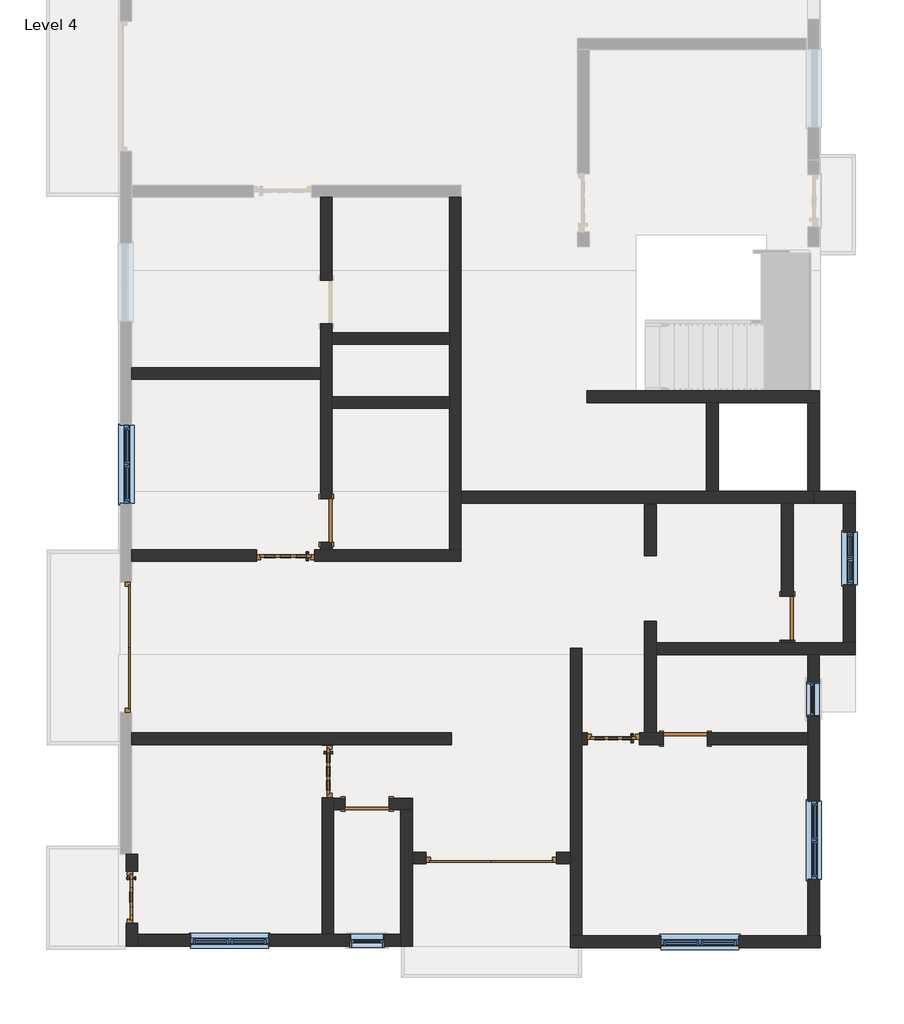
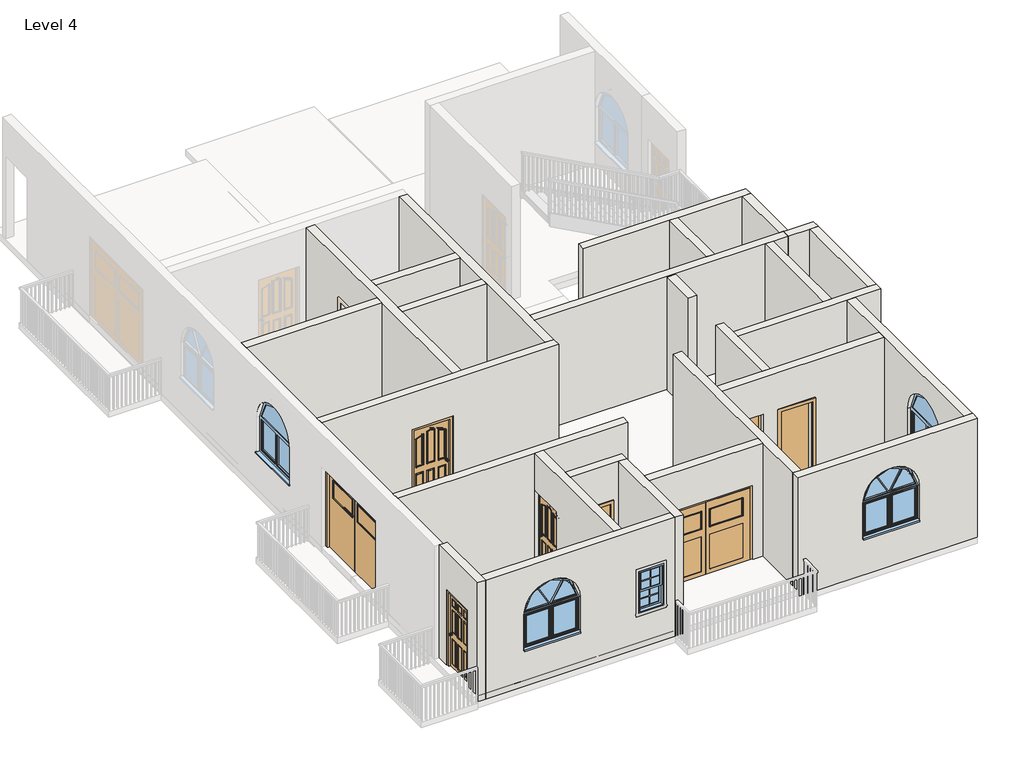
# One storey, part 1 of 7: 27 walls, 10 doors, 7 windows.
"""IFC4 building model written with IfcOpenShell, lengths in millimetres."""

from ifc_helpers import new_model, si_unit, frame, origin, place, context, project, spatial, polyline, circle_curve, outline, extrude, faceted_brep, transform, mapped, element, save
from ifc_brep_helpers import plane_surface, revolved_surface, advanced_brep
from components import doors_extsgl_5_910x2110mm_99758a98, doors_extsgl_6_1010x2110mm_b93c615f, doors_extsgl_6_1010x2110mm_efbaf1af, doors_extsgl_6_910x2110mm_72be2df1, doors_extsgl_6_910x2110mm_b26fcae4, doors_extsgl_6_910x2110mm_5dc58899, doors_extsgl_6_910x2110mm_16d7c084, doors_garage_timber_side_hung_glazing_2270x2050mm_ae99176d, doors_garage_timber_side_hung_glazing_2270x2200mm_badb7014, door_fadea3f2, door_53b1b562, window_679d2811, windows_arched_1360x910mm_c5754810, windows_dbl_w_glazing_bars_910x910mm_41eba874

model = new_model("IFC4")

# Units and contexts
model_context = context("Model", 3, world=origin())
ifc_project = project(units=[si_unit("LENGTHUNIT", "METRE", prefix="MILLI")], contexts=[model_context])

# Site, building, storey
site = spatial("IfcSite", under=ifc_project)
building = spatial("IfcBuilding", under=site)
storey = spatial("IfcBuildingStorey", under=building, Name="Level 4", Elevation=9144.0)

# Doors
placement = place(None, origin())
doors_extsgl_5_910x2110mm_shape = doors_extsgl_5_910x2110mm_99758a98(model_context)
element("IfcDoor", 1, ObjectType="Doors_ExtSgl_5 : 910x2110mm", at=placement, inside=storey, context=model_context, shape_type="MappedRepresentation", body=[
    mapped(doors_extsgl_5_910x2110mm_shape, transform((-6127.6013636, -9759.5108149, 9144.0), x_axis=(0.0, -1.0, 0.0), y_axis=(1.0, 0.0, 0.0), z_axis=(0.0, 0.0, 1.0))),
])
doors_extsgl_6_1010x2110mm_shape = doors_extsgl_6_1010x2110mm_b93c615f(model_context)
doors_extsgl_6_1010x2110mm_2_shape = doors_extsgl_6_1010x2110mm_efbaf1af(model_context)
element("IfcDoor", 2, ObjectType="Doors_ExtSgl_6 : 1010x2110mm", at=placement, inside=storey, context=model_context, shape_type="MappedRepresentation", body=[
    mapped(doors_extsgl_6_1010x2110mm_shape, transform((-3445.8775704, -3805.7037749, 9144.0), x_axis=(-1.0, 0.0, 0.0), y_axis=(0.0, -1.0, 0.0), z_axis=(0.0, 0.0, 1.0))),
    mapped(doors_extsgl_6_1010x2110mm_2_shape, transform((-3445.8775704, -3805.7037749, 9144.0), x_axis=(-1.0, 0.0, 0.0), y_axis=(0.0, -1.0, 0.0), z_axis=(0.0, 0.0, 1.0))),
])
doors_extsgl_6_910x2110mm_shape = doors_extsgl_6_910x2110mm_72be2df1(model_context)
doors_extsgl_6_910x2110mm_2_shape = doors_extsgl_6_910x2110mm_b26fcae4(model_context)
element("IfcDoor", 3, ObjectType="Doors_ExtSgl_6 : 910x2110mm", at=placement, inside=storey, context=model_context, shape_type="MappedRepresentation", body=[
    mapped(doors_extsgl_6_910x2110mm_shape, transform((2269.1224296, -6998.5466225, 9144.0), x_axis=(-1.0, 0.0, 0.0), y_axis=(0.0, -1.0, 0.0), z_axis=(0.0, 0.0, 1.0))),
    mapped(doors_extsgl_6_910x2110mm_2_shape, transform((2269.1224296, -6998.5466225, 9144.0), x_axis=(-1.0, 0.0, 0.0), y_axis=(0.0, -1.0, 0.0), z_axis=(0.0, 0.0, 1.0))),
])
doors_extsgl_6_910x2110mm_3_shape = doors_extsgl_6_910x2110mm_5dc58899(model_context)
doors_extsgl_6_910x2110mm_4_shape = doors_extsgl_6_910x2110mm_16d7c084(model_context)
element("IfcDoor", 4, ObjectType="Doors_ExtSgl_6 : 910x2110mm", at=placement, inside=storey, context=model_context, shape_type="MappedRepresentation", body=[
    mapped(doors_extsgl_6_910x2110mm_3_shape, transform((-2709.3109037, -7568.3747197, 9144.0), x_axis=(0.0, -1.0, 0.0), y_axis=(1.0, 0.0, 0.0), z_axis=(0.0, 0.0, 1.0))),
    mapped(doors_extsgl_6_910x2110mm_4_shape, transform((-2709.3109037, -7568.3747197, 9144.0), x_axis=(0.0, -1.0, 0.0), y_axis=(1.0, 0.0, 0.0), z_axis=(0.0, 0.0, 1.0))),
])
doors_garage_timber_side_hung_glazing_2270x2050mm_shape = doors_garage_timber_side_hung_glazing_2270x2050mm_ae99176d(model_context)
element("IfcDoor", 5, ObjectType="Doors_Garage_Timber_Side_Hung_Glazing : 2270x2050mm", at=placement, inside=storey, context=model_context, shape_type="MappedRepresentation", body=[
    mapped(doors_garage_timber_side_hung_glazing_2270x2050mm_shape, transform((141.8390963, -9078.0694836, 9144.0), x_axis=(-1.0, 0.0, 0.0), y_axis=(0.0, -1.0, 0.0), z_axis=(0.0, 0.0, 1.0))),
])
doors_garage_timber_side_hung_glazing_2270x2200mm_shape = doors_garage_timber_side_hung_glazing_2270x2200mm_badb7014(model_context)
element("IfcDoor", 6, ObjectType="Doors_Garage_Timber_Side_Hung_Glazing : 2270x2200mm", at=placement, inside=storey, context=model_context, shape_type="MappedRepresentation", body=[
    mapped(doors_garage_timber_side_hung_glazing_2270x2200mm_shape, transform((-6229.2013636, -5402.1251987, 9144.0), x_axis=(0.0, 1.0, 0.0), y_axis=(-1.0, 0.0, 0.0), z_axis=(0.0, 0.0, 1.0))),
])
door_shape = door_fadea3f2(model_context)
element("IfcDoor", 7, ObjectType="Single-Flush : 30\" x 80\"", at=placement, inside=storey, context=model_context, shape_type="MappedRepresentation", body=[
    mapped(door_shape, transform((-2023.5109037, -8138.2694836, 9144.0), x_axis=(-1.0, 0.0, 0.0), y_axis=(0.0, -1.0, 0.0), z_axis=(0.0, 0.0, 1.0))),
])
element("IfcDoor", 8, ObjectType="Single-Flush : 30\" x 80\"", at=placement, inside=storey, context=model_context, shape_type="MappedRepresentation", body=[
    mapped(door_shape, transform((5304.3890963, -4897.9037749, 9144.0), x_axis=(0.0, -1.0, 0.0), y_axis=(1.0, 0.0, 0.0), z_axis=(0.0, 0.0, 1.0))),
])
door_2_shape = door_53b1b562(model_context)
element("IfcDoor", 9, ObjectType="Single-Flush : 30\" x 80\"", at=placement, inside=storey, context=model_context, shape_type="MappedRepresentation", body=[
    mapped(door_2_shape, transform((-2734.7109037, -3196.1037749, 9144.0), x_axis=(0.0, 1.0, 0.0), y_axis=(-1.0, 0.0, 0.0), z_axis=(0.0, 0.0, 1.0))),
])
element("IfcDoor", 10, ObjectType="Single-Flush : 30\" x 80\"", at=placement, inside=storey, context=model_context, shape_type="MappedRepresentation", body=[
    mapped(door_2_shape, transform((3526.3890963, -6998.5466225, 9144.0), x_axis=(-1.0, 0.0, 0.0), y_axis=(0.0, -1.0, 0.0), z_axis=(0.0, 0.0, 1.0))),
])

# Walls
element("IfcWall", 11, ObjectType="Generic - 9\" w", at=placement, inside=storey, context=model_context, shape_type="Brep", body=[
    faceted_brep([(6485.4890963, -2688.1037749, 9144.0), (5863.1890963, -2688.1037749, 9144.0), (5761.5890963, -2688.1037749, 9144.0), (5761.5890963, -2688.1037749, 12192.0), (5863.1890963, -2688.1037749, 12192.0), (6485.4890963, -2688.1037749, 12192.0), (6485.4890963, -2891.3037749, 9144.0), (6485.4890963, -2891.3037749, 12192.0), (6282.2890963, -2891.3037749, 12192.0), (5761.5890963, -2891.3037749, 12192.0), (5761.5890963, -2891.3037749, 9144.0), (6282.2890963, -2891.3037749, 9144.0)], [[[0, 1, 2, 3, 4, 5]], [[6, 7, 8, 9, 10, 11]], [[2, 1, 0, 6, 11, 10]], [[3, 2, 10, 9]], [[5, 4, 3, 9, 8, 7]], [[0, 5, 7, 6]]]),
])
element("IfcWall", 12, ObjectType="Generic - 9\" w", at=placement, inside=storey, context=model_context, shape_type="Brep", body=[
    faceted_brep([(5761.5890963, -2688.1037749, 9144.0), (5659.9890963, -2688.1037749, 9144.0), (4097.8890963, -2688.1037749, 9144.0), (3894.6890963, -2688.1037749, 9144.0), (-385.2109037, -2688.1037749, 9144.0), (-385.2109037, -2688.1037749, 12192.0), (3894.6890963, -2688.1037749, 12192.0), (4097.8890963, -2688.1037749, 12192.0), (5659.9890963, -2688.1037749, 12192.0), (5761.5890963, -2688.1037749, 12192.0), (5761.5890963, -2891.3037749, 9144.0), (5761.5890963, -2891.3037749, 12192.0), (5405.9890963, -2891.3037749, 12192.0), (5202.7890963, -2891.3037749, 12192.0), (-385.2109037, -2891.3037749, 12192.0), (-385.2109037, -2891.3037749, 9144.0), (5202.7890963, -2891.3037749, 9144.0), (5405.9890963, -2891.3037749, 9144.0)], [[[0, 1, 2, 3, 4, 5, 6, 7, 8, 9]], [[10, 11, 12, 13, 14, 15, 16, 17]], [[4, 3, 2, 1, 0, 10, 17, 16, 15]], [[9, 8, 7, 6, 5, 14, 13, 12, 11]], [[0, 9, 11, 10]], [[5, 4, 15, 14]]]),
])
element("IfcWall", 13, ObjectType="Generic - 9\" w", at=placement, inside=storey, context=model_context, shape_type="SweptSolid", body=[
    extrude(outline(polyline([(3894.6890963, -2688.1037749), (3894.6890963, -1138.7037749), (4097.8890963, -1138.7037749), (4097.8890963, -2688.1037749), (3894.6890963, -2688.1037749)])), frame((0.0, 0.0, 9144.0), z_axis=(0.0, 0.0, 1.0), x_axis=(1.0, 0.0, 0.0)), (0.0, 0.0, 1.0), 3048.0),
])
element("IfcWall", 14, ObjectType="Generic - 9\" w", at=placement, inside=storey, context=model_context, shape_type="Brep", body=[
    faceted_brep([(5863.1890963, -935.5037749, 9144.0), (1812.4805171, -935.5037749, 9144.0), (1812.4805171, -935.5037749, 12192.0), (5863.1890963, -935.5037749, 12192.0), (5863.1890963, -1138.7037749, 9144.0), (5863.1890963, -1138.7037749, 12192.0), (5659.9890963, -1138.7037749, 12192.0), (4097.8890963, -1138.7037749, 12192.0), (3894.6890963, -1138.7037749, 12192.0), (1812.4805171, -1138.7037749, 12192.0), (1812.4805171, -1138.7037749, 9144.0), (3894.6890963, -1138.7037749, 9144.0), (4097.8890963, -1138.7037749, 9144.0), (5659.9890963, -1138.7037749, 9144.0)], [[[0, 1, 2, 3]], [[4, 5, 6, 7, 8, 9, 10, 11, 12, 13]], [[1, 0, 4, 13, 12, 11, 10]], [[2, 1, 10, 9]], [[3, 2, 9, 8, 7, 6, 5]], [[0, 3, 5, 4]]]),
])
element("IfcWall", 15, ObjectType="Generic - 9\" w", at=placement, inside=storey, context=model_context, shape_type="AdvancedBrep", body=[
    advanced_brep(
    [(1519.7890963, -10638.3037749, 9144.0), (5875.8890963, -10638.3037749, 9144.0), (5875.8890963, -10638.3037749, 12192.0), (1519.7890963, -10638.3037749, 12192.0), (4460.3890963, -10638.3037749, 10058.4), (3100.3890963, -10638.3037749, 10058.4), (3100.3890963, -10638.3037749, 10968.4), (4460.3890963, -10638.3037749, 10968.4), (1519.7890963, -10435.1037749, 9144.0), (1519.7890963, -10435.1037749, 12192.0), (1722.9890963, -10435.1037749, 12192.0), (5659.9890963, -10435.1037749, 12192.0), (5863.1890963, -10435.1037749, 12192.0), (5875.8890963, -10435.1037749, 12192.0), (5875.8890963, -10435.1037749, 9144.0), (5863.1890963, -10435.1037749, 9144.0), (5659.9890963, -10435.1037749, 9144.0), (1722.9890963, -10435.1037749, 9144.0), (4460.3890963, -10435.1037749, 10058.4), (4460.3890963, -10435.1037749, 10968.4), (3100.3890963, -10435.1037749, 10968.4), (3100.3890963, -10435.1037749, 10058.4)],
    [
        (0, 1),
        (1, 2),
        (2, 3),
        (3, 0),
        (4, 5),
        (5, 6),
        (6, 7, circle_curve(frame((3780.3890963, -10638.3037749, 10968.4), z_axis=(0.0, 1.0, 0.0), x_axis=(-1.0, 0.0, 0.0)), 680.0)),
        (7, 4),
        (8, 9),
        (9, 10),
        (10, 11),
        (11, 12),
        (12, 13),
        (13, 14),
        (14, 15),
        (15, 16),
        (16, 17),
        (17, 8),
        (18, 19),
        (19, 20, circle_curve(frame((3780.3890963, -10435.1037749, 10968.4), z_axis=(0.0, -1.0, 0.0), x_axis=(-1.0, 0.0, 0.0)), 680.0)),
        (20, 21),
        (21, 18),
        (0, 8),
        (14, 1),
        (13, 2),
        (9, 3),
        (18, 4),
        (7, 19),
        (6, 20),
        (5, 21),
    ],
    [
        plane_surface(frame((1722.9890963, -10638.3037749, 9144.0), z_axis=(0.0, -1.0, 0.0), x_axis=(1.0, 0.0, 0.0))),
        plane_surface(frame((1722.9890963, -10435.1037749, 9144.0), z_axis=(0.0, 1.0, 0.0), x_axis=(-1.0, 0.0, 0.0))),
        plane_surface(frame((1621.3890963, -10638.3037749, 9144.0), z_axis=(0.0, 0.0, -1.0), x_axis=(0.0, 1.0, 0.0))),
        plane_surface(frame((5875.8890963, -10638.3037749, 9144.0), z_axis=(1.0, 0.0, 0.0), x_axis=(0.0, 1.0, 0.0))),
        plane_surface(frame((5875.8890963, -10638.3037749, 12192.0), z_axis=(0.0, 0.0, 1.0), x_axis=(0.0, 1.0, 0.0))),
        plane_surface(frame((1519.7890963, -5418.6037749, 9144.0), z_axis=(-1.0, 0.0, 0.0), x_axis=(0.0, -1.0, 0.0))),
        plane_surface(frame((4460.3890963, -10435.1037749, 10058.4), z_axis=(-1.0, 0.0, 0.0), x_axis=(0.0, -1.0, 0.0))),
        revolved_surface(polyline([(3100.3890963, -10638.3037749, 10968.4), (3100.3890963, -10435.1037749, 10968.4)]), (3780.3890963, -10435.1037749, 10968.4), (0.0, -1.0, 0.0)),
        plane_surface(frame((3100.3890963, -10435.1037749, 10968.4), z_axis=(1.0, 0.0, 0.0), x_axis=(0.0, -1.0, 0.0))),
        plane_surface(frame((3100.3890963, -10435.1037749, 10058.4), z_axis=(0.0, 0.0, 1.0), x_axis=(0.0, -1.0, 0.0))),
    ],
    [
        (0, [[1, 2, 3, 4], [5, 6, 7, 8]]),
        (1, [[9, 10, 11, 12, 13, 14, 15, 16, 17, 18], [19, 20, 21, 22]]),
        (2, [[-1, 23, -18, -17, -16, -15, 24]]),
        (3, [[-2, -24, -14, 25]]),
        (4, [[-3, -25, -13, -12, -11, -10, 26]]),
        (5, [[-4, -26, -9, -23]]),
        (6, [[-19, 27, -8, 28]]),
        (7, [[-20, -28, -7, 29]]),
        (8, [[-21, -29, -6, 30]]),
        (9, [[-22, -30, -5, -27]]),
    ],
),
])
element("IfcWall", 16, ObjectType="Generic - 9\" w", at=placement, inside=storey, context=model_context, shape_type="AdvancedBrep", body=[
    advanced_brep(
    [(5863.1890963, -10435.1037749, 9144.0), (5863.1890963, -5532.9037749, 9144.0), (5863.1890963, -5532.9037749, 12192.0), (5863.1890963, -10435.1037749, 12192.0), (5863.1890963, -8087.6251987, 10058.4), (5863.1890963, -9447.6251987, 10058.4), (5863.1890963, -9447.6251987, 10968.4), (5863.1890963, -8087.6251987, 10968.4), (5863.1890963, -6618.7537749, 11125.2), (5863.1890963, -6009.1537749, 11125.2), (5863.1890963, -6009.1537749, 10058.4), (5863.1890963, -6618.7537749, 10058.4), (5659.9890963, -10435.1037749, 9144.0), (5659.9890963, -10435.1037749, 12192.0), (5659.9890963, -7100.1466225, 12192.0), (5659.9890963, -6896.9466225, 12192.0), (5659.9890963, -5532.9037749, 12192.0), (5659.9890963, -5532.9037749, 9144.0), (5659.9890963, -6896.9466225, 9144.0), (5659.9890963, -7100.1466225, 9144.0), (5659.9890963, -8087.6251987, 10058.4), (5659.9890963, -8087.6251987, 10968.4), (5659.9890963, -9447.6251987, 10968.4), (5659.9890963, -9447.6251987, 10058.4), (5659.9890963, -6618.7537749, 11125.2), (5659.9890963, -6618.7537749, 10058.4), (5659.9890963, -6009.1537749, 10058.4), (5659.9890963, -6009.1537749, 11125.2)],
    [
        (0, 1),
        (1, 2),
        (2, 3),
        (3, 0),
        (4, 5),
        (5, 6),
        (6, 7, circle_curve(frame((5863.1890963, -8767.6251987, 10968.4), z_axis=(-1.0, 0.0, 0.0), x_axis=(0.0, -1.0, 0.0)), 680.0)),
        (7, 4),
        (8, 9),
        (9, 10),
        (10, 11),
        (11, 8),
        (12, 13),
        (13, 14),
        (14, 15),
        (15, 16),
        (16, 17),
        (17, 18),
        (18, 19),
        (19, 12),
        (20, 21),
        (21, 22, circle_curve(frame((5659.9890963, -8767.6251987, 10968.4), z_axis=(1.0, 0.0, 0.0), x_axis=(0.0, -1.0, 0.0)), 680.0)),
        (22, 23),
        (23, 20),
        (24, 25),
        (25, 26),
        (26, 27),
        (27, 24),
        (0, 12),
        (17, 1),
        (2, 16),
        (13, 3),
        (20, 4),
        (7, 21),
        (6, 22),
        (5, 23),
        (24, 8),
        (11, 25),
        (10, 26),
        (9, 27),
    ],
    [
        plane_surface(frame((5863.1890963, -10435.1037749, 9144.0), z_axis=(1.0, 0.0, 0.0), x_axis=(0.0, 1.0, 0.0))),
        plane_surface(frame((5659.9890963, -10435.1037749, 9144.0), z_axis=(-1.0, 0.0, 0.0), x_axis=(0.0, -1.0, 0.0))),
        plane_surface(frame((5863.1890963, -10536.7037749, 9144.0), z_axis=(0.0, 0.0, -1.0), x_axis=(-1.0, 0.0, 0.0))),
        plane_surface(frame((5863.1890963, -5431.3037749, 12192.0), z_axis=(0.0, 0.0, 1.0), x_axis=(-1.0, 0.0, 0.0))),
        plane_surface(frame((1722.9890963, -10435.1037749, 9144.0), z_axis=(0.0, -1.0, 0.0), x_axis=(-1.0, 0.0, 0.0))),
        plane_surface(frame((3018.3890963, -5532.9037749, 9144.0), z_axis=(0.0, 1.0, 0.0), x_axis=(1.0, 0.0, 0.0))),
        plane_surface(frame((5659.9890963, -8087.6251987, 10058.4), z_axis=(0.0, -1.0, 0.0), x_axis=(1.0, 0.0, 0.0))),
        revolved_surface(polyline([(5863.1890963, -9447.6251987, 10968.4), (5659.9890963, -9447.6251987, 10968.4)]), (5659.9890963, -8767.6251987, 10968.4), (1.0, 0.0, 0.0)),
        plane_surface(frame((5659.9890963, -9447.6251987, 10968.4), z_axis=(0.0, 1.0, 0.0), x_axis=(1.0, 0.0, 0.0))),
        plane_surface(frame((5659.9890963, -9447.6251987, 10058.4), z_axis=(0.0, 0.0, 1.0), x_axis=(1.0, 0.0, 0.0))),
        plane_surface(frame((5659.9890963, -6618.7537749, 11125.2), z_axis=(0.0, 1.0, 0.0), x_axis=(1.0, 0.0, 0.0))),
        plane_surface(frame((5659.9890963, -6618.7537749, 10058.4), z_axis=(0.0, 0.0, 1.0), x_axis=(1.0, 0.0, 0.0))),
        plane_surface(frame((5659.9890963, -6009.1537749, 10058.4), z_axis=(0.0, -1.0, 0.0), x_axis=(1.0, 0.0, 0.0))),
        plane_surface(frame((5659.9890963, -6009.1537749, 11125.2), z_axis=(0.0, 0.0, -1.0), x_axis=(1.0, 0.0, 0.0))),
    ],
    [
        (0, [[1, 2, 3, 4], [5, 6, 7, 8], [9, 10, 11, 12]]),
        (1, [[13, 14, 15, 16, 17, 18, 19, 20], [21, 22, 23, 24], [25, 26, 27, 28]]),
        (2, [[-1, 29, -20, -19, -18, 30]]),
        (3, [[-3, 31, -16, -15, -14, 32]]),
        (4, [[-4, -32, -13, -29]]),
        (5, [[-2, -30, -17, -31]]),
        (6, [[-21, 33, -8, 34]]),
        (7, [[-22, -34, -7, 35]]),
        (8, [[-23, -35, -6, 36]]),
        (9, [[-24, -36, -5, -33]]),
        (10, [[-25, 37, -12, 38]]),
        (11, [[-26, -38, -11, 39]]),
        (12, [[-27, -39, -10, 40]]),
        (13, [[-28, -40, -9, -37]]),
    ],
),
])
element("IfcWall", 17, ObjectType="Generic - 9\" w", at=placement, inside=storey, context=model_context, shape_type="Brep", body=[
    faceted_brep([(5659.9890963, -1138.7037749, 9144.0), (5659.9890963, -2688.1037749, 9144.0), (5659.9890963, -2688.1037749, 12192.0), (5659.9890963, -1138.7037749, 12192.0), (5863.1890963, -1138.7037749, 9144.0), (5863.1890963, -1138.7037749, 12192.0), (5863.1890963, -2688.1037749, 12192.0), (5863.1890963, -2688.1037749, 9144.0), (5761.5890963, -2688.1037749, 9144.0), (5761.5890963, -2688.1037749, 12192.0)], [[[0, 1, 2, 3]], [[4, 5, 6, 7]], [[1, 0, 4, 7, 8]], [[3, 2, 9, 6, 5]], [[2, 1, 8, 7, 6, 9]], [[0, 3, 5, 4]]]),
])
element("IfcWall", 18, ObjectType="Generic - 9\" w", at=placement, inside=storey, context=model_context, shape_type="Brep", body=[
    faceted_brep([(-6229.2013636, -10214.5441482, 11254.0), (-6229.2013636, -10214.5441482, 9144.0), (-6229.2013636, -10612.9037749, 9144.0), (-6229.2013636, -10612.9037749, 12192.0), (-6229.2013636, -9007.7845215, 12192.0), (-6229.2013636, -9007.7845215, 9144.0), (-6229.2013636, -9304.5441482, 9144.0), (-6229.2013636, -9304.5441482, 11254.0), (-6026.0013636, -10612.9037749, 9144.0), (-6026.0013636, -10409.7037749, 9144.0), (-6026.0013636, -10214.5441482, 9144.0), (-6026.0013636, -10214.5441482, 11254.0), (-6026.0013636, -9304.5441482, 11254.0), (-6026.0013636, -9304.5441482, 9144.0), (-6026.0013636, -9007.7845215, 9144.0), (-6026.0013636, -9007.7845215, 12192.0), (-6026.0013636, -10409.7037749, 12192.0), (-6026.0013636, -10612.9037749, 12192.0), (-6127.6013636, -9007.7845215, 9144.0), (-6127.6013636, -9007.7845215, 12192.0)], [[[0, 1, 2, 3, 4, 5, 6, 7]], [[8, 9, 10, 11, 12, 13, 14, 15, 16, 17]], [[6, 5, 18, 14, 13]], [[2, 1, 10, 9, 8]], [[4, 3, 17, 16, 15, 19]], [[5, 4, 19, 15, 14, 18]], [[13, 12, 7, 6]], [[11, 10, 1, 0]], [[12, 11, 0, 7]], [[3, 2, 8, 17]]]),
])
element("IfcWall", 19, ObjectType="Generic - 9\" w", at=placement, inside=storey, context=model_context, shape_type="AdvancedBrep", body=[
    advanced_brep(
    [(-6026.0013636, -10612.9037749, 9144.0), (-1439.3109037, -10612.9037749, 9144.0), (-1439.3109037, -10612.9037749, 12192.0), (-6026.0013636, -10612.9037749, 12192.0), (-3738.4561337, -10612.9037749, 10058.4), (-5098.4561337, -10612.9037749, 10058.4), (-5098.4561337, -10612.9037749, 10968.4), (-3738.4561337, -10612.9037749, 10968.4), (-1718.7109037, -10612.9037749, 11125.2), (-1718.7109037, -10612.9037749, 10058.4), (-2328.3109037, -10612.9037749, 10058.4), (-2328.3109037, -10612.9037749, 11125.2), (-6026.0013636, -10409.7037749, 9144.0), (-6026.0013636, -10409.7037749, 12192.0), (-2810.9109037, -10409.7037749, 12192.0), (-2607.7109037, -10409.7037749, 12192.0), (-1439.3109037, -10409.7037749, 12192.0), (-1439.3109037, -10409.7037749, 9144.0), (-2607.7109037, -10409.7037749, 9144.0), (-2810.9109037, -10409.7037749, 9144.0), (-3738.4561337, -10409.7037749, 10058.4), (-3738.4561337, -10409.7037749, 10968.4), (-5098.4561337, -10409.7037749, 10968.4), (-5098.4561337, -10409.7037749, 10058.4), (-1718.7109037, -10409.7037749, 11125.2), (-2328.3109037, -10409.7037749, 11125.2), (-2328.3109037, -10409.7037749, 10058.4), (-1718.7109037, -10409.7037749, 10058.4)],
    [
        (0, 1),
        (1, 2),
        (2, 3),
        (3, 0),
        (4, 5),
        (5, 6),
        (6, 7, circle_curve(frame((-4418.4561337, -10612.9037749, 10968.4), z_axis=(0.0, 1.0, 0.0), x_axis=(-1.0, 0.0, 0.0)), 680.0)),
        (7, 4),
        (8, 9),
        (9, 10),
        (10, 11),
        (11, 8),
        (12, 13),
        (13, 14),
        (14, 15),
        (15, 16),
        (16, 17),
        (17, 18),
        (18, 19),
        (19, 12),
        (20, 21),
        (21, 22, circle_curve(frame((-4418.4561337, -10409.7037749, 10968.4), z_axis=(0.0, -1.0, 0.0), x_axis=(-1.0, 0.0, 0.0)), 680.0)),
        (22, 23),
        (23, 20),
        (24, 25),
        (25, 26),
        (26, 27),
        (27, 24),
        (0, 12),
        (17, 1),
        (2, 16),
        (13, 3),
        (20, 4),
        (7, 21),
        (6, 22),
        (5, 23),
        (8, 24),
        (27, 9),
        (26, 10),
        (25, 11),
    ],
    [
        plane_surface(frame((-6229.2013636, -10612.9037749, 9144.0), z_axis=(0.0, -1.0, 0.0), x_axis=(1.0, 0.0, 0.0))),
        plane_surface(frame((-6229.2013636, -10409.7037749, 9144.0), z_axis=(0.0, 1.0, 0.0), x_axis=(-1.0, 0.0, 0.0))),
        plane_surface(frame((-6127.6013636, -10612.9037749, 9144.0), z_axis=(0.0, 0.0, -1.0), x_axis=(0.0, 1.0, 0.0))),
        plane_surface(frame((-1337.7109037, -10612.9037749, 12192.0), z_axis=(0.0, 0.0, 1.0), x_axis=(0.0, 1.0, 0.0))),
        plane_surface(frame((-1439.3109037, -8239.8694836, 9144.0), z_axis=(1.0, 0.0, 0.0), x_axis=(0.0, -1.0, 0.0))),
        plane_surface(frame((-6026.0013636, -9109.3845215, 9144.0), z_axis=(-1.0, 0.0, 0.0), x_axis=(0.0, 1.0, 0.0))),
        plane_surface(frame((-3738.4561337, -10409.7037749, 10058.4), z_axis=(-1.0, 0.0, 0.0), x_axis=(0.0, -1.0, 0.0))),
        revolved_surface(polyline([(-5098.4561337, -10612.9037749, 10968.4), (-5098.4561337, -10409.7037749, 10968.4)]), (-4418.4561337, -10409.7037749, 10968.4), (0.0, -1.0, 0.0)),
        plane_surface(frame((-5098.4561337, -10409.7037749, 10968.4), z_axis=(1.0, 0.0, 0.0), x_axis=(0.0, -1.0, 0.0))),
        plane_surface(frame((-5098.4561337, -10409.7037749, 10058.4), z_axis=(0.0, 0.0, 1.0), x_axis=(0.0, -1.0, 0.0))),
        plane_surface(frame((-1718.7109037, -10612.9037749, 11125.2), z_axis=(-1.0, 0.0, 0.0), x_axis=(0.0, 1.0, 0.0))),
        plane_surface(frame((-1718.7109037, -10612.9037749, 10058.4), z_axis=(0.0, 0.0, 1.0), x_axis=(0.0, 1.0, 0.0))),
        plane_surface(frame((-2328.3109037, -10612.9037749, 10058.4), z_axis=(1.0, 0.0, 0.0), x_axis=(0.0, 1.0, 0.0))),
        plane_surface(frame((-2328.3109037, -10612.9037749, 11125.2), z_axis=(0.0, 0.0, -1.0), x_axis=(0.0, 1.0, 0.0))),
    ],
    [
        (0, [[1, 2, 3, 4], [5, 6, 7, 8], [9, 10, 11, 12]]),
        (1, [[13, 14, 15, 16, 17, 18, 19, 20], [21, 22, 23, 24], [25, 26, 27, 28]]),
        (2, [[-1, 29, -20, -19, -18, 30]]),
        (3, [[-3, 31, -16, -15, -14, 32]]),
        (4, [[-2, -30, -17, -31]]),
        (5, [[-4, -32, -13, -29]]),
        (6, [[-21, 33, -8, 34]]),
        (7, [[-22, -34, -7, 35]]),
        (8, [[-23, -35, -6, 36]]),
        (9, [[-24, -36, -5, -33]]),
        (10, [[-9, 37, -28, 38]]),
        (11, [[-10, -38, -27, 39]]),
        (12, [[-11, -39, -26, 40]]),
        (13, [[-12, -40, -25, -37]]),
    ],
),
])
element("IfcWall", 20, ObjectType="Generic -4.5\" p", at=placement, inside=storey, context=model_context, shape_type="Brep", body=[
    faceted_brep([(-2836.3109037, 232.8962251, 9144.0), (-2836.3109037, -529.1037749, 9144.0), (-2836.3109037, -732.3037749, 9144.0), (-2836.3109037, -2815.1037749, 9144.0), (-2836.3109037, -2815.1037749, 11176.0), (-2836.3109037, -3577.1037749, 11176.0), (-2836.3109037, -3577.1037749, 9144.0), (-2836.3109037, -3704.1037749, 9144.0), (-2836.3109037, -3704.1037749, 12192.0), (-2836.3109037, -732.3037749, 12192.0), (-2836.3109037, -529.1037749, 12192.0), (-2836.3109037, 2442.6962251, 12192.0), (-2836.3109037, 2442.6962251, 9144.0), (-2836.3109037, 994.8962251, 9144.0), (-2836.3109037, 994.8962251, 11176.0), (-2836.3109037, 232.8962251, 11176.0), (-2633.1109037, -2815.1037749, 11176.0), (-2633.1109037, -2815.1037749, 9144.0), (-2633.1109037, -1240.3037749, 9144.0), (-2633.1109037, -1037.1037749, 9144.0), (-2633.1109037, -122.7037749, 9144.0), (-2633.1109037, 80.4962251, 9144.0), (-2633.1109037, 232.8962251, 9144.0), (-2633.1109037, 232.8962251, 11176.0), (-2633.1109037, 994.8962251, 11176.0), (-2633.1109037, 994.8962251, 9144.0), (-2633.1109037, 2442.6962251, 9144.0), (-2633.1109037, 2442.6962251, 12192.0), (-2633.1109037, 80.4962251, 12192.0), (-2633.1109037, -122.7037749, 12192.0), (-2633.1109037, -1037.1037749, 12192.0), (-2633.1109037, -1240.3037749, 12192.0), (-2633.1109037, -3704.1037749, 12192.0), (-2633.1109037, -3704.1037749, 9144.0), (-2633.1109037, -3577.1037749, 9144.0), (-2633.1109037, -3577.1037749, 11176.0)], [[[0, 1, 2, 3, 4, 5, 6, 7, 8, 9, 10, 11, 12, 13, 14, 15]], [[16, 17, 18, 19, 20, 21, 22, 23, 24, 25, 26, 27, 28, 29, 30, 31, 32, 33, 34, 35]], [[26, 25, 13, 12]], [[34, 33, 7, 6]], [[22, 21, 20, 19, 18, 17, 3, 2, 1, 0]], [[11, 10, 9, 8, 32, 31, 30, 29, 28, 27]], [[12, 11, 27, 26]], [[8, 7, 33, 32]], [[14, 13, 25, 24]], [[15, 14, 24, 23]], [[0, 15, 23, 22]], [[4, 3, 17, 16]], [[5, 4, 16, 35]], [[6, 5, 35, 34]]]),
])
element("IfcWall", 21, ObjectType="Generic -4.5\" p", at=placement, inside=storey, context=model_context, shape_type="Brep", body=[
    faceted_brep([(-6127.6013636, -3907.3037749, 9144.0), (-3950.9109037, -3907.3037749, 9144.0), (-3950.9109037, -3907.3037749, 11254.0), (-2940.9109037, -3907.3037749, 11254.0), (-2940.9109037, -3907.3037749, 9144.0), (-385.2109037, -3907.3037749, 9144.0), (-385.2109037, -3907.3037749, 12192.0), (-6127.6013636, -3907.3037749, 12192.0), (-3950.9109037, -3704.1037749, 11254.0), (-3950.9109037, -3704.1037749, 9144.0), (-6127.6013636, -3704.1037749, 9144.0), (-6127.6013636, -3704.1037749, 12192.0), (-2836.3109037, -3704.1037749, 12192.0), (-2633.1109037, -3704.1037749, 12192.0), (-588.4109037, -3704.1037749, 12192.0), (-385.2109037, -3704.1037749, 12192.0), (-385.2109037, -3704.1037749, 9144.0), (-588.4109037, -3704.1037749, 9144.0), (-2633.1109037, -3704.1037749, 9144.0), (-2836.3109037, -3704.1037749, 9144.0), (-2940.9109037, -3704.1037749, 9144.0), (-2940.9109037, -3704.1037749, 11254.0)], [[[0, 1, 2, 3, 4, 5, 6, 7]], [[8, 9, 10, 11, 12, 13, 14, 15, 16, 17, 18, 19, 20, 21]], [[10, 9, 1, 0]], [[20, 19, 18, 17, 16, 5, 4]], [[7, 6, 15, 14, 13, 12, 11]], [[6, 5, 16, 15]], [[4, 3, 21, 20]], [[2, 1, 9, 8]], [[3, 2, 8, 21]], [[0, 7, 11, 10]]]),
])
element("IfcWall", 22, ObjectType="Generic -4.5\" p", at=placement, inside=storey, context=model_context, shape_type="Brep", body=[
    faceted_brep([(-385.2109037, -3704.1037749, 9144.0), (-385.2109037, -2891.3037749, 9144.0), (-385.2109037, -2688.1037749, 9144.0), (-385.2109037, 2442.6962251, 9144.0), (-385.2109037, 2442.6962251, 12192.0), (-385.2109037, -2688.1037749, 12192.0), (-385.2109037, -2891.3037749, 12192.0), (-385.2109037, -3704.1037749, 12192.0), (-588.4109037, -3704.1037749, 9144.0), (-588.4109037, -3704.1037749, 12192.0), (-588.4109037, -1240.3037749, 12192.0), (-588.4109037, -1037.1037749, 12192.0), (-588.4109037, -122.7037749, 12192.0), (-588.4109037, 80.4962251, 12192.0), (-588.4109037, 2442.6962251, 12192.0), (-588.4109037, 2442.6962251, 9144.0), (-588.4109037, 80.4962251, 9144.0), (-588.4109037, -122.7037749, 9144.0), (-588.4109037, -1037.1037749, 9144.0), (-588.4109037, -1240.3037749, 9144.0)], [[[0, 1, 2, 3, 4, 5, 6, 7]], [[8, 9, 10, 11, 12, 13, 14, 15, 16, 17, 18, 19]], [[3, 2, 1, 0, 8, 19, 18, 17, 16, 15]], [[7, 6, 5, 4, 14, 13, 12, 11, 10, 9]], [[4, 3, 15, 14]], [[0, 7, 9, 8]]]),
])
element("IfcWall", 23, ObjectType="Generic -4.5\" p", at=placement, inside=storey, context=model_context, shape_type="SweptSolid", body=[
    extrude(outline(polyline([(-588.4109037, -122.7037749), (-2633.1109037, -122.7037749), (-2633.1109037, 80.4962251), (-588.4109037, 80.4962251), (-588.4109037, -122.7037749)])), frame((0.0, 0.0, 9144.0), z_axis=(0.0, 0.0, 1.0), x_axis=(1.0, 0.0, 0.0)), (0.0, 0.0, 1.0), 3048.0),
])
element("IfcWall", 24, ObjectType="Generic -4.5\" p", at=placement, inside=storey, context=model_context, shape_type="SweptSolid", body=[
    extrude(outline(polyline([(-2836.3109037, -732.3037749), (-6127.6013636, -732.3037749), (-6127.6013636, -529.1037749), (-2836.3109037, -529.1037749), (-2836.3109037, -732.3037749)])), frame((0.0, 0.0, 9144.0), z_axis=(0.0, 0.0, 1.0), x_axis=(1.0, 0.0, 0.0)), (0.0, 0.0, 1.0), 3048.0),
])
element("IfcWall", 25, ObjectType="Generic -4.5\" p", at=placement, inside=storey, context=model_context, shape_type="SweptSolid", body=[
    extrude(outline(polyline([(-588.4109037, -1240.3037749), (-2633.1109037, -1240.3037749), (-2633.1109037, -1037.1037749), (-588.4109037, -1037.1037749), (-588.4109037, -1240.3037749)])), frame((0.0, 0.0, 9144.0), z_axis=(0.0, 0.0, 1.0), x_axis=(1.0, 0.0, 0.0)), (0.0, 0.0, 1.0), 3048.0),
])
element("IfcWall", 26, ObjectType="Generic -4.5\" p", at=placement, inside=storey, context=model_context, shape_type="Brep", body=[
    faceted_brep([(-6127.6013636, -7100.1466225, 9144.0), (-2810.9109037, -7100.1466225, 9144.0), (-2607.7109037, -7100.1466225, 9144.0), (-550.3109037, -7100.1466225, 9144.0), (-550.3109037, -7100.1466225, 12192.0), (-2607.7109037, -7100.1466225, 12192.0), (-2810.9109037, -7100.1466225, 12192.0), (-6127.6013636, -7100.1466225, 12192.0), (-6127.6013636, -6896.9466225, 9144.0), (-6127.6013636, -6896.9466225, 12192.0), (-550.3109037, -6896.9466225, 12192.0), (-550.3109037, -6896.9466225, 9144.0)], [[[0, 1, 2, 3, 4, 5, 6, 7]], [[8, 9, 10, 11]], [[3, 2, 1, 0, 8, 11]], [[4, 3, 11, 10]], [[7, 6, 5, 4, 10, 9]], [[0, 7, 9, 8]]]),
])
element("IfcWall", 27, ObjectType="Generic -4.5\" p", at=placement, inside=storey, context=model_context, shape_type="Brep", body=[
    faceted_brep([(-2607.7109037, -10409.7037749, 9144.0), (-2607.7109037, -8239.8694836, 9144.0), (-2607.7109037, -8036.6694836, 9144.0), (-2607.7109037, -8023.4080531, 9144.0), (-2607.7109037, -8023.4080531, 11254.0), (-2607.7109037, -7113.4080531, 11254.0), (-2607.7109037, -7113.4080531, 9144.0), (-2607.7109037, -7100.1466225, 9144.0), (-2607.7109037, -7100.1466225, 12192.0), (-2607.7109037, -8036.6694836, 12192.0), (-2607.7109037, -8239.8694836, 12192.0), (-2607.7109037, -10409.7037749, 12192.0), (-2810.9109037, -8023.4080531, 11254.0), (-2810.9109037, -8023.4080531, 9144.0), (-2810.9109037, -10409.7037749, 9144.0), (-2810.9109037, -10409.7037749, 12192.0), (-2810.9109037, -7100.1466225, 12192.0), (-2810.9109037, -7100.1466225, 9144.0), (-2810.9109037, -7113.4080531, 9144.0), (-2810.9109037, -7113.4080531, 11254.0)], [[[0, 1, 2, 3, 4, 5, 6, 7, 8, 9, 10, 11]], [[12, 13, 14, 15, 16, 17, 18, 19]], [[18, 17, 7, 6]], [[14, 13, 3, 2, 1, 0]], [[11, 10, 9, 8, 16, 15]], [[8, 7, 17, 16]], [[6, 5, 19, 18]], [[4, 3, 13, 12]], [[5, 4, 12, 19]], [[0, 11, 15, 14]]]),
])
element("IfcWall", 28, ObjectType="Generic -4.5\" p", at=placement, inside=storey, context=model_context, shape_type="Brep", body=[
    faceted_brep([(-2607.7109037, -8239.8694836, 9144.0), (-2404.5109037, -8239.8694836, 9144.0), (-2404.5109037, -8239.8694836, 11176.0), (-1642.5109037, -8239.8694836, 11176.0), (-1642.5109037, -8239.8694836, 9144.0), (-1439.3109037, -8239.8694836, 9144.0), (-1236.1109037, -8239.8694836, 9144.0), (-1236.1109037, -8239.8694836, 12192.0), (-1439.3109037, -8239.8694836, 12192.0), (-2607.7109037, -8239.8694836, 12192.0), (-2404.5109037, -8036.6694836, 11176.0), (-2404.5109037, -8036.6694836, 9144.0), (-2607.7109037, -8036.6694836, 9144.0), (-2607.7109037, -8036.6694836, 12192.0), (-1236.1109037, -8036.6694836, 12192.0), (-1236.1109037, -8036.6694836, 9144.0), (-1642.5109037, -8036.6694836, 9144.0), (-1642.5109037, -8036.6694836, 11176.0)], [[[0, 1, 2, 3, 4, 5, 6, 7, 8, 9]], [[10, 11, 12, 13, 14, 15, 16, 17]], [[16, 15, 6, 5, 4]], [[12, 11, 1, 0]], [[9, 8, 7, 14, 13]], [[0, 9, 13, 12]], [[7, 6, 15, 14]], [[2, 1, 11, 10]], [[3, 2, 10, 17]], [[4, 3, 17, 16]]]),
])
element("IfcWall", 29, ObjectType="Generic -4.5\" p", at=placement, inside=storey, context=model_context, shape_type="Brep", body=[
    faceted_brep([(-1439.3109037, -8239.8694836, 9144.0), (-1439.3109037, -10409.7037749, 9144.0), (-1439.3109037, -10612.9037749, 9144.0), (-1439.3109037, -10612.9037749, 12192.0), (-1439.3109037, -10409.7037749, 12192.0), (-1439.3109037, -8239.8694836, 12192.0), (-1236.1109037, -8239.8694836, 9144.0), (-1236.1109037, -8239.8694836, 12192.0), (-1236.1109037, -8976.4694836, 12192.0), (-1236.1109037, -9179.6694836, 12192.0), (-1236.1109037, -10612.9037749, 12192.0), (-1236.1109037, -10612.9037749, 9144.0), (-1236.1109037, -9179.6694836, 9144.0), (-1236.1109037, -8976.4694836, 9144.0)], [[[0, 1, 2, 3, 4, 5]], [[6, 7, 8, 9, 10, 11, 12, 13]], [[2, 1, 0, 6, 13, 12, 11]], [[5, 4, 3, 10, 9, 8, 7]], [[3, 2, 11, 10]], [[0, 5, 7, 6]]]),
])
element("IfcWall", 30, ObjectType="Generic -4.5\" p", at=placement, inside=storey, context=model_context, shape_type="SweptSolid", body=[
    extrude(outline(polyline([(9144.0, -1236.1109037), (9144.0, -993.1609037), (11194.0, -993.1609037), (11194.0, 1276.8390963), (9144.0, 1276.8390963), (9144.0, 1519.7890963), (12192.0, 1519.7890963), (12192.0, -1236.1109037), (9144.0, -1236.1109037)])), frame((0.0, -9179.6694836, 0.0), z_axis=(0.0, 1.0, 0.0), x_axis=(0.0, 0.0, 1.0)), (0.0, 0.0, 1.0), 203.2),
])
element("IfcWall", 31, ObjectType="Generic -4.5\" p", at=placement, inside=storey, context=model_context, shape_type="Brep", body=[
    faceted_brep([(1519.7890963, -5418.6037749, 9144.0), (1519.7890963, -8976.4694836, 9144.0), (1519.7890963, -9179.6694836, 9144.0), (1519.7890963, -10435.1037749, 9144.0), (1519.7890963, -10435.1037749, 12192.0), (1519.7890963, -9179.6694836, 12192.0), (1519.7890963, -8976.4694836, 12192.0), (1519.7890963, -5418.6037749, 12192.0), (1722.9890963, -5418.6037749, 9144.0), (1722.9890963, -5418.6037749, 12192.0), (1722.9890963, -6896.9466225, 12192.0), (1722.9890963, -7100.1466225, 12192.0), (1722.9890963, -10435.1037749, 12192.0), (1722.9890963, -10435.1037749, 9144.0), (1722.9890963, -7100.1466225, 9144.0), (1722.9890963, -6896.9466225, 9144.0)], [[[0, 1, 2, 3, 4, 5, 6, 7]], [[8, 9, 10, 11, 12, 13, 14, 15]], [[3, 2, 1, 0, 8, 15, 14, 13]], [[7, 6, 5, 4, 12, 11, 10, 9]], [[0, 7, 9, 8]], [[4, 3, 13, 12]]]),
])
element("IfcWall", 32, ObjectType="Generic -4.5\" p", at=placement, inside=storey, context=model_context, shape_type="Brep", body=[
    faceted_brep([(2724.0890963, -7100.1466225, 9144.0), (3145.3890963, -7100.1466225, 9144.0), (3145.3890963, -7100.1466225, 11176.0), (3907.3890963, -7100.1466225, 11176.0), (3907.3890963, -7100.1466225, 9144.0), (5659.9890963, -7100.1466225, 9144.0), (5659.9890963, -7100.1466225, 12192.0), (1722.9890963, -7100.1466225, 12192.0), (1722.9890963, -7100.1466225, 9144.0), (1814.0890963, -7100.1466225, 9144.0), (1814.0890963, -7100.1466225, 11254.0), (2724.0890963, -7100.1466225, 11254.0), (3145.3890963, -6896.9466225, 11176.0), (3145.3890963, -6896.9466225, 9144.0), (3018.3890963, -6896.9466225, 9144.0), (2815.1890963, -6896.9466225, 9144.0), (2724.0890963, -6896.9466225, 9144.0), (2724.0890963, -6896.9466225, 11254.0), (1814.0890963, -6896.9466225, 11254.0), (1814.0890963, -6896.9466225, 9144.0), (1722.9890963, -6896.9466225, 9144.0), (1722.9890963, -6896.9466225, 12192.0), (2815.1890963, -6896.9466225, 12192.0), (3018.3890963, -6896.9466225, 12192.0), (5659.9890963, -6896.9466225, 12192.0), (5659.9890963, -6896.9466225, 9144.0), (3907.3890963, -6896.9466225, 9144.0), (3907.3890963, -6896.9466225, 11176.0)], [[[0, 1, 2, 3, 4, 5, 6, 7, 8, 9, 10, 11]], [[12, 13, 14, 15, 16, 17, 18, 19, 20, 21, 22, 23, 24, 25, 26, 27]], [[20, 19, 9, 8]], [[26, 25, 5, 4]], [[16, 15, 14, 13, 1, 0]], [[7, 6, 24, 23, 22, 21]], [[6, 5, 25, 24]], [[8, 7, 21, 20]], [[0, 11, 17, 16]], [[10, 9, 19, 18]], [[11, 10, 18, 17]], [[2, 1, 13, 12]], [[3, 2, 12, 27]], [[4, 3, 27, 26]]]),
])
element("IfcWall", 33, ObjectType="Generic -4.5\" p", at=placement, inside=storey, context=model_context, shape_type="Brep", body=[
    faceted_brep([(3018.3890963, -6896.9466225, 9144.0), (3018.3890963, -5532.9037749, 9144.0), (3018.3890963, -5329.7037749, 9144.0), (3018.3890963, -4949.7445151, 9144.0), (3018.3890963, -4949.7445151, 12192.0), (3018.3890963, -5329.7037749, 12192.0), (3018.3890963, -5532.9037749, 12192.0), (3018.3890963, -6896.9466225, 12192.0), (2815.1890963, -6896.9466225, 9144.0), (2815.1890963, -6896.9466225, 12192.0), (2815.1890963, -4949.7445151, 12192.0), (2815.1890963, -4949.7445151, 9144.0)], [[[0, 1, 2, 3, 4, 5, 6, 7]], [[8, 9, 10, 11]], [[3, 2, 1, 0, 8, 11]], [[4, 3, 11, 10]], [[7, 6, 5, 4, 10, 9]], [[0, 7, 9, 8]]]),
])
element("IfcWall", 34, ObjectType="Generic -4.5\" p", at=placement, inside=storey, context=model_context, shape_type="Brep", body=[
    faceted_brep([(3018.3890963, -5532.9037749, 9144.0), (5659.9890963, -5532.9037749, 9144.0), (5863.1890963, -5532.9037749, 9144.0), (6485.4890963, -5532.9037749, 9144.0), (6485.4890963, -5532.9037749, 12192.0), (5863.1890963, -5532.9037749, 12192.0), (5659.9890963, -5532.9037749, 12192.0), (3018.3890963, -5532.9037749, 12192.0), (3018.3890963, -5329.7037749, 9144.0), (3018.3890963, -5329.7037749, 12192.0), (5202.7890963, -5329.7037749, 12192.0), (5405.9890963, -5329.7037749, 12192.0), (6282.2890963, -5329.7037749, 12192.0), (6485.4890963, -5329.7037749, 12192.0), (6485.4890963, -5329.7037749, 9144.0), (6282.2890963, -5329.7037749, 9144.0), (5405.9890963, -5329.7037749, 9144.0), (5202.7890963, -5329.7037749, 9144.0)], [[[0, 1, 2, 3, 4, 5, 6, 7]], [[8, 9, 10, 11, 12, 13, 14, 15, 16, 17]], [[3, 2, 1, 0, 8, 17, 16, 15, 14]], [[7, 6, 5, 4, 13, 12, 11, 10, 9]], [[0, 7, 9, 8]], [[4, 3, 14, 13]]]),
])
element("IfcWall", 35, ObjectType="Generic -4.5\" p", at=placement, inside=storey, context=model_context, shape_type="SweptSolid", body=[
    extrude(outline(polyline([(-5329.7037749, 9144.0), (-5329.7037749, 12192.0), (-2891.3037749, 12192.0), (-2891.3037749, 9144.0), (-5329.7037749, 9144.0)]), holes=[polyline([(-3401.5037749, 10968.4), (-4311.5037749, 10968.4), (-4311.5037749, 10058.4), (-3401.5037749, 10058.4), (-3401.5037749, 10968.4)])]), frame((6282.2890963, 0.0, 0.0), z_axis=(1.0, 0.0, 0.0), x_axis=(0.0, 1.0, 0.0)), (0.0, 0.0, 1.0), 203.2),
])
element("IfcWall", 36, ObjectType="Generic -4.5\" p", at=placement, inside=storey, context=model_context, shape_type="SweptSolid", body=[
    extrude(outline(polyline([(-5278.9037749, 11176.0), (-5278.9037749, 9144.0), (-5329.7037749, 9144.0), (-5329.7037749, 12192.0), (-2891.3037749, 12192.0), (-2891.3037749, 9144.0), (-4516.9037749, 9144.0), (-4516.9037749, 11176.0), (-5278.9037749, 11176.0)])), frame((5202.7890963, 0.0, 0.0), z_axis=(1.0, 0.0, 0.0), x_axis=(0.0, 1.0, 0.0)), (0.0, 0.0, 1.0), 203.2),
])
element("IfcWall", 37, ObjectType="Generic -4.5\" p", at=placement, inside=storey, context=model_context, shape_type="SweptSolid", body=[
    extrude(outline(polyline([(2815.1890963, -3808.4464026), (2815.1890963, -2916.7037749), (3018.3890963, -2916.7037749), (3018.3890963, -3808.4464026), (2815.1890963, -3808.4464026)])), frame((0.0, 0.0, 9144.0), z_axis=(0.0, 0.0, 1.0), x_axis=(1.0, 0.0, 0.0)), (0.0, 0.0, 1.0), 3048.0),
])

# Windows
window_shape = window_679d2811(model_context)
element("IfcWindow", 38, ObjectType="Window-Double-Hung : 24\" x 42\"", at=placement, inside=storey, context=model_context, shape_type="MappedRepresentation", body=[
    mapped(window_shape, transform((5761.5890963, -6313.9537749, 9144.0), x_axis=(0.0, 1.0, 0.0), y_axis=(-1.0, 0.0, 0.0), z_axis=(0.0, 0.0, 1.0))),
])
element("IfcWindow", 39, ObjectType="Window-Double-Hung : 24\" x 42\"", at=placement, inside=storey, context=model_context, shape_type="MappedRepresentation", body=[
    mapped(window_shape, transform((-2023.5109037, -10511.3037749, 9144.0), x_axis=(-1.0, 0.0, 0.0), y_axis=(0.0, -1.0, 0.0), z_axis=(0.0, 0.0, 1.0))),
])
windows_arched_1360x910mm_shape = windows_arched_1360x910mm_c5754810(model_context)
element("IfcWindow", 40, ObjectType="Windows_Arched : 1360x910mm", at=placement, inside=storey, context=model_context, shape_type="MappedRepresentation", body=[
    mapped(windows_arched_1360x910mm_shape, transform((-6237.6579314, -2503.2037749, 8858.4), x_axis=(0.0, -1.0, 0.0), y_axis=(1.0, 0.0, 0.0), z_axis=(0.0, 0.0, 1.0))),
])
element("IfcWindow", 41, ObjectType="Windows_Arched : 1360x910mm", at=placement, inside=storey, context=model_context, shape_type="MappedRepresentation", body=[
    mapped(windows_arched_1360x910mm_shape, transform((5753.1325284, -9052.6251987, 8858.4), x_axis=(0.0, -1.0, 0.0), y_axis=(1.0, 0.0, 0.0), z_axis=(0.0, 0.0, 1.0))),
])
element("IfcWindow", 42, ObjectType="Windows_Arched : 1360x910mm", at=placement, inside=storey, context=model_context, shape_type="MappedRepresentation", body=[
    mapped(windows_arched_1360x910mm_shape, transform((3495.3890963, -10528.2472071, 8858.4), x_axis=(-1.0, 0.0, 0.0), y_axis=(0.0, -1.0, 0.0), z_axis=(0.0, 0.0, 1.0))),
])
element("IfcWindow", 43, ObjectType="Windows_Arched : 1360x910mm", at=placement, inside=storey, context=model_context, shape_type="MappedRepresentation", body=[
    mapped(windows_arched_1360x910mm_shape, transform((-4703.4561337, -10502.8472071, 8858.4), x_axis=(-1.0, 0.0, 0.0), y_axis=(0.0, -1.0, 0.0), z_axis=(0.0, 0.0, 1.0))),
])
windows_dbl_w_glazing_bars_910x910mm_shape = windows_dbl_w_glazing_bars_910x910mm_41eba874(model_context)
element("IfcWindow", 44, ObjectType="Windows_Dbl_w-Glazing_Bars : 910x910mm", at=placement, inside=storey, context=model_context, shape_type="MappedRepresentation", body=[
    mapped(windows_dbl_w_glazing_bars_910x910mm_shape, transform((6375.4325284, -3986.5037749, 8868.4), x_axis=(0.0, -1.0, 0.0), y_axis=(1.0, 0.0, 0.0), z_axis=(0.0, 0.0, 1.0))),
])

save(model, "model.ifc")

# Revit data of these elements
# Type "Doors_ExtSgl_5 : 910x2110mm"
#   Type Mark = "11"
#   Type Comments = "External Single"
#   Operation = "SingleSwingRight"
#   Construction Type Id = "MDOOR"
#   Keynote = "L20"
#   Analytic Construction = "Metal"
#   Wrap Layers (Int) from Ext = 0' - 6.98819"
#   Wrap Layers (Ext) from Ext = 0' - 4.03543"
#   Thickness = 0' - 1.73228"
#   Stile Top of Lock rail = 3' - 3.37008"
#   Stile Top of Frieze Rail = 5' - 4.96063"
#   Stile Top Rail = 0' - 5.90551"
#   Stile Shutting = 0' - 3.14961"
#   Stile Muntin Rail = 0' - 2.95276"
#   Stile Lock Rail = 0' - 6.88976"
#   Stile Intermediate/Frieze = 0' - 3.14961"
#   Stile Hanging = 0' - 3.14961"
#   Stile Bottom Rail = 0' - 6.88976"
#   Rough Width = 2' - 11.82677"
#   Rough Height = 6' - 11.07087"
#   O/A Frame Width = 0' - 2.51969"
#   Heat Transfer Coefficient (U) = 0.651978 BTU/(h·ft²·°F)
#   Handle Z Distance = 3' - 3.37008"
#   Glazing Thickness = 0' - 0.94488"
#   FrameWidth = 0' - 1.65354"
#   FrameOffset - External = 0' - 0.98425"
#   FrameDepth = 0' - 3.50394"
#   Door Panel Width = 2' - 7.77165"
#   Door Panel Thickness = 0' - 1.73228"
#   Door Panel Height = 6' - 6.74016"
#   DONT CHANGE - Panel Width = 0' - 6.52231"
#   Cill Thickness = 0' - 2.14567"
#   Cill Projection = 0' - 1.1811"
#   Handle X Distance = 0' - 2.95276"
#   Height = 6' - 11.07087"
#   Structural Tolerance = 0' - 0.25591"
#   Tolerance = 0' - 0.11811"
#   Undercut = 0' - 0.15748"
#   Width = 2' - 11.82677"
#   Cill Extension = 0' - 0.98425"
#   Cavity Closer Width = 0' - 1.9685"
#   Cavity Closer Offset from Ext = 0' - 4.03543"
#   Cavity Closer Depth = 0' - 3.34646"
#   Vis - Ironmongery = yes
#   Vis - Cavity Closers = yes
#   Define Thermal Properties by = 1
#   Function = 1
#   Material Glass = Door - Glazing
#   Material Door = Door - Panel
#   Material Frame = Door - Frame/Mullion
#   Material Ironmongery = Door - Handle
#   Visual Light Transmittance = 0
#   Solar Heat Gain Coefficient = 0
#   Wall Closure = (empty or 0)
# Type "Doors_ExtSgl_6 : 1010x2110mm"
#   Type Mark = "12"
#   Type Comments = "External Single"
#   Operation = "SingleSwingRight"
#   Construction Type Id = "SGL"
#   Keynote = "L20"
#   Analytic Construction = "Large single-glazed windows"
#   Wrap Layers (Int) from Ext = 0' - 6.98819"
#   Wrap Layers (Ext) from Ext = 0' - 4.03543"
#   Visual Light Transmittance = 0.9
#   Thickness = 0' - 1.73228"
#   Stile Top of Lock rail = 3' - 3.37008"
#   Stile Top Rail = 0' - 5.90551"
#   Stile Shutting = 0' - 3.54331"
#   Stile Muntin Rail = 0' - 3.54331"
#   Stile Lock Rail = 0' - 6.88976"
#   Stile Hanging = 0' - 3.54331"
#   Stile Bottom Rail = 0' - 6.88976"
#   Solar Heat Gain Coefficient = 0.86
#   Rough Width = 3' - 3.76378"
#   Rough Height = 6' - 11.07087"
#   O/A Frame Width = 0' - 2.51969"
#   Heat Transfer Coefficient (U) = 0.979472 BTU/(h·ft²·°F)
#   Handle Z Distance = 3' - 3.37008"
#   Glazing Thickness = 0' - 0.94488"
#   FrameWidth = 0' - 1.65354"
#   FrameOffset - External = 0' - 0.98425"
#   FrameDepth = 0' - 3.50394"
#   Door Panel Width = 2' - 11.70866"
#   Door Panel Thickness = 0' - 1.73228"
#   Door Panel Height = 6' - 6.74016"
#   DONT CHANGE - Panel Width = 0' - 7.17848"
#   Cill Thickness = 0' - 2.14567"
#   Cill Projection = 0' - 1.1811"
#   Handle X Distance = 0' - 2.95276"
#   Height = 6' - 11.07087"
#   Structural Tolerance = 0' - 0.25591"
#   Tolerance = 0' - 0.11811"
#   Undercut = 0' - 0.15748"
#   Width = 3' - 3.76378"
#   Cill Extension = 0' - 0.98425"
#   Cavity Closer Width = 0' - 1.9685"
#   Cavity Closer Offset from Ext = 0' - 4.03543"
#   Cavity Closer Depth = 0' - 3.34646"
#   Vis - Ironmongery = yes
#   Vis - Cavity Closers = yes
#   Define Thermal Properties by = 1
#   Function = 1
#   Material Glass = Door - Glazing
#   Material Door = Door - Panel
#   Material Frame = Door - Frame/Mullion
#   Material Ironmongery = Door - Handle
#   Wall Closure = (empty or 0)
# Type "Doors_ExtSgl_6 : 910x2110mm"
#   Type Mark = "13"
#   Type Comments = "External Single"
#   Operation = "SingleSwingRight"
#   Construction Type Id = "SGL"
#   Keynote = "L20"
#   Analytic Construction = "Large single-glazed windows"
#   Wrap Layers (Int) from Ext = 0' - 6.98819"
#   Wrap Layers (Ext) from Ext = 0' - 4.03543"
#   Visual Light Transmittance = 0.9
#   Thickness = 0' - 1.73228"
#   Stile Top of Lock rail = 3' - 3.37008"
#   Stile Top Rail = 0' - 5.90551"
#   Stile Shutting = 0' - 3.14961"
#   Stile Muntin Rail = 0' - 2.95276"
#   Stile Lock Rail = 0' - 6.88976"
#   Stile Hanging = 0' - 3.14961"
#   Stile Bottom Rail = 0' - 6.88976"
#   Solar Heat Gain Coefficient = 0.86
#   Rough Width = 2' - 11.82677"
#   Rough Height = 6' - 11.07087"
#   O/A Frame Width = 0' - 2.51969"
#   Heat Transfer Coefficient (U) = 0.979472 BTU/(h·ft²·°F)
#   Handle Z Distance = 3' - 3.37008"
#   Glazing Thickness = 0' - 0.94488"
#   FrameWidth = 0' - 1.65354"
#   FrameOffset - External = 0' - 0.98425"
#   FrameDepth = 0' - 3.50394"
#   Door Panel Width = 2' - 7.77165"
#   Door Panel Thickness = 0' - 1.73228"
#   Door Panel Height = 6' - 6.74016"
#   DONT CHANGE - Panel Width = 0' - 6.52231"
#   Cill Thickness = 0' - 2.14567"
#   Cill Projection = 0' - 1.1811"
#   Handle X Distance = 0' - 2.95276"
#   Height = 6' - 11.07087"
#   Structural Tolerance = 0' - 0.25591"
#   Tolerance = 0' - 0.11811"
#   Undercut = 0' - 0.15748"
#   Width = 2' - 11.82677"
#   Cill Extension = 0' - 0.98425"
#   Cavity Closer Width = 0' - 1.9685"
#   Cavity Closer Offset from Ext = 0' - 4.03543"
#   Cavity Closer Depth = 0' - 3.34646"
#   Vis - Ironmongery = yes
#   Vis - Cavity Closers = yes
#   Define Thermal Properties by = 1
#   Function = 1
#   Material Glass = Door - Glazing
#   Material Door = Door - Panel
#   Material Frame = Door - Frame/Mullion
#   Material Ironmongery = Door - Handle
#   Wall Closure = (empty or 0)
# Type "Doors_Garage_Timber_Side_Hung_Glazing : 2270x2050mm"
#   Type Mark = "8"
#   Type Comments = "External Garage"
#   Operation = "DoubleDoorSingleSwing"
#   Construction Type Id = "GSP4R"
#   Manufacturer = "Revit"
#   Keynote = "L20"
#   Analytic Construction = "1/8 in Pilkington single glazing"
#   Wrap Layers (Ext) from Ext = 0' - 4.03543"
#   Wrap Layers (Int) from Ext = 0' - 6.98819"
#   Visual Light Transmittance = 0.9
#   Thickness = 0' - 1.25984"
#   Stile Top Rail = 0' - 7.87402"
#   Stile Shutting = 0' - 3.93701"
#   Stile Lock Rail = 0' - 7.87402"
#   Stile Hanging = 0' - 6.88976"
#   Stile Bottom Rail = 0' - 9.84252"
#   Solar Heat Gain Coefficient = 0.78
#   Rough Width = 7' - 5.37008"
#   Rough Height = 6' - 8.70866"
#   O/A Frame Width = 0' - 2.51969"
#   Heat Transfer Coefficient (U) = 0.6496 BTU/(h·ft²·°F)
#   Handle Z Distance = 3' - 5.33858"
#   Glazing Panel Height = 1' - 5.71654"
#   FrameWidth = 0' - 1.65354"
#   FrameOffset - External = 0' - 0.98425"
#   FrameDepth = 0' - 3.50394"
#   Door Panel Thickness = 0' - 1.25984"
#   Height = 6' - 8.70866"
#   Structural Tolerance = 0' - 0.31496"
#   Tolerance = 0' - 0.11811"
#   Undercut = 0' - 0.3937"
#   Width = 7' - 5.37008"
#   Cavity Closer Width = 0' - 1.9685"
#   Cavity Closer Offset from Ext = 0' - 4.03543"
#   Cavity Closer Depth = 0' - 3.34646"
#   Vis - Cavity Closers = yes
#   Define Thermal Properties by = 1
#   Function = 1
#   Material Door = Door - Panel
#   Material Frame = Door - Frame/Mullion
#   Material Ironmongery = Door - Handle
#   Wall Closure = (empty or 0)
# Type "Doors_Garage_Timber_Side_Hung_Glazing : 2270x2200mm"
#   Type Mark = "9"
#   Type Comments = "External Garage"
#   Operation = "DoubleDoorSingleSwing"
#   Construction Type Id = "GSP4R"
#   Manufacturer = "Revit"
#   Keynote = "L20"
#   Analytic Construction = "1/8 in Pilkington single glazing"
#   Wrap Layers (Ext) from Ext = 0' - 4.03543"
#   Wrap Layers (Int) from Ext = 0' - 6.98819"
#   Visual Light Transmittance = 0.9
#   Thickness = 0' - 1.25984"
#   Stile Top Rail = 0' - 7.87402"
#   Stile Shutting = 0' - 3.93701"
#   Stile Lock Rail = 0' - 7.87402"
#   Stile Hanging = 0' - 6.88976"
#   Stile Bottom Rail = 0' - 9.84252"
#   Solar Heat Gain Coefficient = 0.78
#   Rough Width = 7' - 5.37008"
#   Rough Height = 7' - 2.61417"
#   O/A Frame Width = 0' - 2.51969"
#   Heat Transfer Coefficient (U) = 0.6496 BTU/(h·ft²·°F)
#   Handle Z Distance = 3' - 5.33858"
#   Glazing Panel Height = 1' - 5.71654"
#   FrameWidth = 0' - 1.65354"
#   FrameOffset - External = 0' - 0.98425"
#   FrameDepth = 0' - 3.50394"
#   Door Panel Thickness = 0' - 1.25984"
#   Height = 7' - 2.61417"
#   Structural Tolerance = 0' - 0.31496"
#   Tolerance = 0' - 0.11811"
#   Undercut = 0' - 0.3937"
#   Width = 7' - 5.37008"
#   Cavity Closer Width = 0' - 1.9685"
#   Cavity Closer Offset from Ext = 0' - 4.03543"
#   Cavity Closer Depth = 0' - 3.34646"
#   Vis - Cavity Closers = yes
#   Define Thermal Properties by = 1
#   Function = 1
#   Material Door = Door - Panel
#   Material Frame = Door - Frame/Mullion
#   Material Ironmongery = Door - Handle
#   Wall Closure = (empty or 0)
# Type "Single-Flush : 30\" x 80\""
#   Type Mark = "5"
